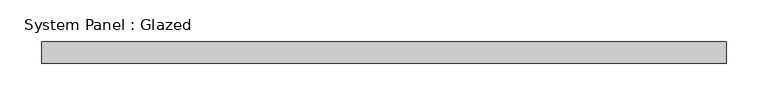
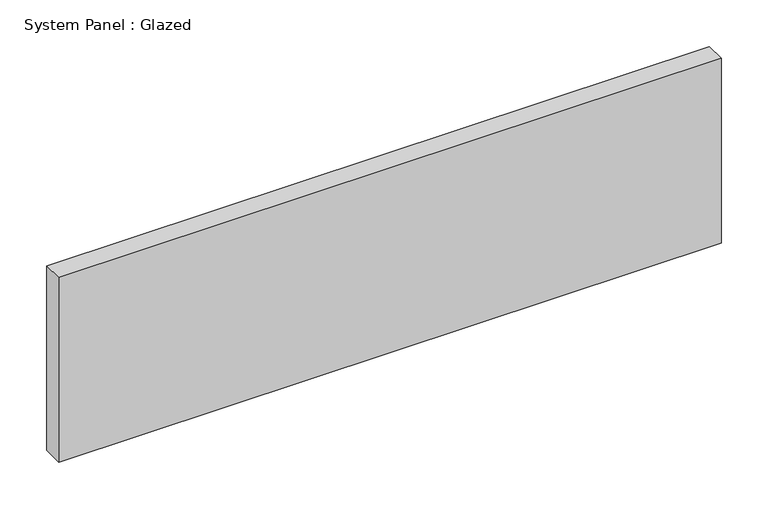
"""IFC4 building model written with IfcOpenShell, lengths in millimetres: plate geometry, System Panel : Glazed."""

from ifc_helpers import new_model, si_unit, origin, origin_with_axes, place, context, project, spatial, polyline, outline, extrude, source, transform, mapped, element, save


def system_panel_glazed_4137532c(model_context):
    return source(origin(), model_context, "Body", "SweptSolid", [
        extrude(outline(polyline([(409.575, 19.05), (-409.575, 19.05), (-409.575, 44.45), (409.575, 44.45), (409.575, 19.05)])), origin_with_axes(), (0.0, 0.0, 1.0), 241.3),
    ])


if __name__ == "__main__":
    model = new_model("IFC4")
    model_context = context("Model", 3, world=origin())
    ifc_project = project(units=[si_unit("LENGTHUNIT", "METRE", prefix="MILLI")], contexts=[model_context])
    site = spatial("IfcSite", under=ifc_project)
    building = spatial("IfcBuilding", under=site)
    placement = place(None, origin())
    system_panel_glazed_shape = system_panel_glazed_4137532c(model_context)
    element("IfcPlate", 1, ObjectType="System Panel : Glazed", at=placement, inside=building, context=model_context, shape_type="MappedRepresentation", body=[
        mapped(system_panel_glazed_shape, transform((0.0, 0.0, 0.0), x_axis=(1.0, 0.0, 0.0), y_axis=(0.0, 1.0, 0.0), z_axis=(0.0, 0.0, 1.0))),
    ])
    save(model, "model.ifc")

# Revit data of these elements
# Type "System Panel : Glazed"
#   Construction Type Id = "GSP4R"
#   Analytic Construction = "1/8 in Pilkington single glazing"
#   Visual Light Transmittance = 0.9
#   Solar Heat Gain Coefficient = 0.86
#   Heat Transfer Coefficient (U) = 6.7069 W/(m²·K)
# Element 1 (IfcPlate, "System Panel : Glazed")
#   Materials on its faces: "Glass"
# Materials
#   "Glass": class "Glass", colour RGB 0 128 192, transparency 0.75, Description = "Soda Lime Glass", Cost = 0
